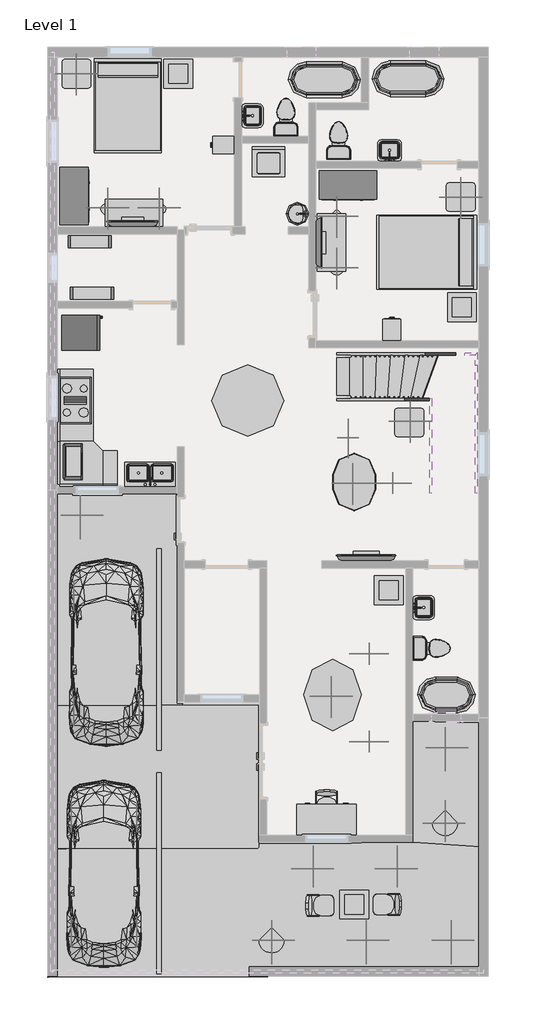
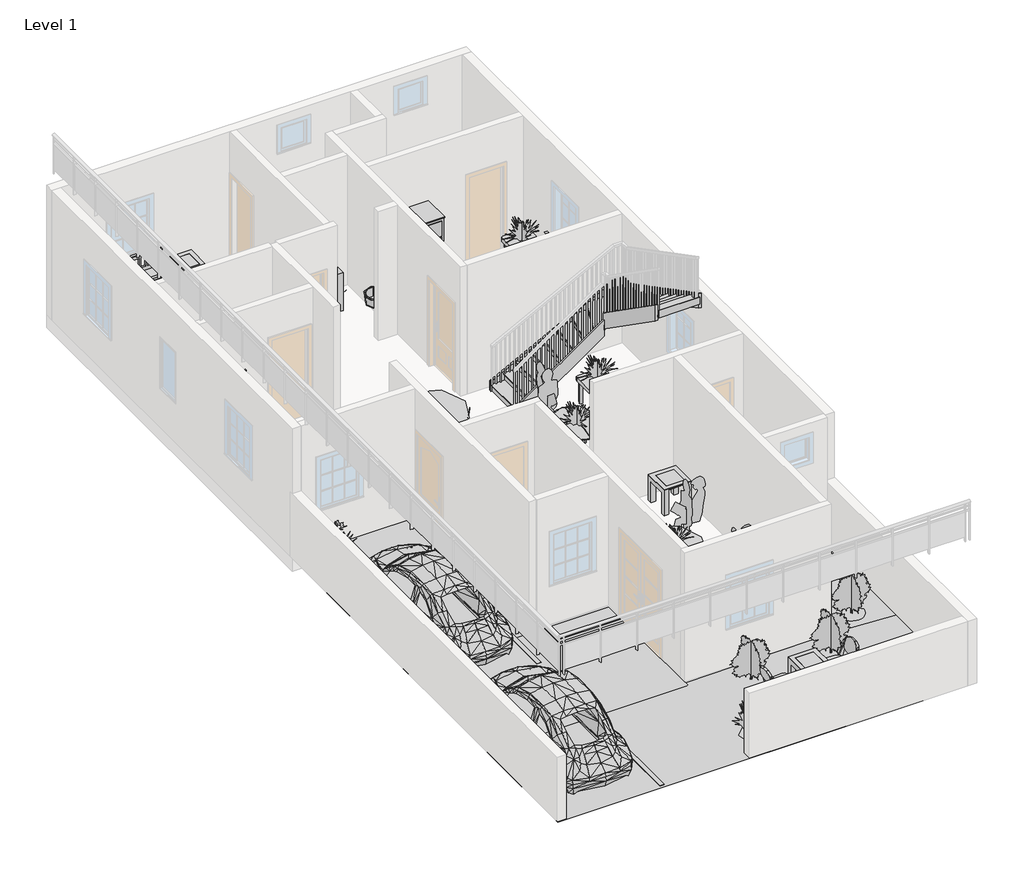
# One storey, part 4 of 4: 28 furniture elements, 17 geographic elements, 16 proxies, 15 flow terminals, 6 members, 1 stair flight.
"""IFC4 building model written with IfcOpenShell, lengths in millimetres."""

from ifc_helpers import new_model, si_unit, frame, origin, place, context, project, spatial, polyline, outline, extrude, triangles, transform, mapped, element, save
from components import proxy_bb1e6e30, proxy_8a8d5ab2, parking_space_9_x_18_90_deg_fdd9e8f5, rpc_beetle_rpc_beetle_3ce7ba48, rpc_female_69e001fa, proxy_a13a33b2, proxy_718fa39f, flow_terminal_accce45a, flow_terminal_a53be723, flow_terminal_d49f872f, flow_terminal_62a433f7, toilet_domestic_3d_toilet_domestic_3d_f7549cf7, toilet_domestic_3d_toilet_domestic_3d_183bbd19, flow_terminal_b374fae2, flow_terminal_04541809, furniture_096e7f55, furniture_35c09872, furniture_bb55ed6b, furniture_e086674a, furniture_9fa109b2, furniture_3d1d9cbc, furniture_417d203a, furniture_7a3aaa4f, furniture_fdf74506, furniture_b5c51a22, furniture_be1c6672, furniture_bbcc68ce, furniture_743965d2, furniture_31d08a24, furniture_9a1a9c00, furniture_823e54a9, rpc_plant_tropical_55f6ff97, rpc_plant_tropical_agave_1_5_93a2a214, rpc_plant_tropical_jungle_flame_3_9c4808c2, stair_flight_aca28aa2

model = new_model("IFC4")

# Units and contexts
model_context = context("Model", 3, world=origin())
ifc_project = project(units=[si_unit("LENGTHUNIT", "METRE", prefix="MILLI")], contexts=[model_context])

# Site, building, storey
site = spatial("IfcSite", under=ifc_project)
building = spatial("IfcBuilding", under=site)
storey = spatial("IfcBuildingStorey", under=building, Name="Level 1", Elevation=0.0)

# Proxies
placement = place(None, origin())
element("IfcBuildingElementProxy", 1, Name="Building Element Proxy", at=placement, inside=storey, context=model_context, shape_type="Tessellation", body=[
    triangles([(-11802.0982178, 4379.0271858, 0.0), (-9058.8976364, 4379.0271858, 0.0), (-9058.8976364, -27.872824, 0.0), (-11802.0982178, -114.4208502, 0.0), (-8906.4976364, -27.872824, 0.0), (-9058.2005859, -225.4422167, 0.0)], [[1, 4, 3], [3, 4, 6], [1, 3, 2], [3, 5, 2], [5, 3, 6]], closed=False),
])
element("IfcBuildingElementProxy", 2, Name="Building Element Proxy", at=placement, inside=storey, context=model_context, shape_type="Tessellation", body=[
    triangles([(-11802.0982178, -3160.0754265, 0.0), (-2454.8975395, -3120.3229111, 0.0), (-2454.8975395, -5857.1727173, 0.0), (-11802.0982178, -5882.5729111, 0.0), (-4069.6108978, -3091.2976479, 0.0), (-7295.5854996, -3097.5405807, 0.0), (-4055.0975395, -3012.3728142, 0.0), (-7312.4141235, -3043.6589859, 0.0)], [[1, 4, 6], [8, 6, 7], [6, 8, 1], [4, 3, 6], [3, 2, 5], [5, 7, 6], [7, 5, 2], [3, 5, 6]], closed=False),
])
element("IfcBuildingElementProxy", 3, Name="Building Element Proxy", at=placement, inside=storey, context=model_context, shape_type="Tessellation", body=[
    triangles([(-11598.8978302, -112.4571982, 0.0), (-11598.8978302, -3148.0770309, 0.0), (-7349.0310745, -187.3552247, 0.0), (-7347.7823135, -3140.2966919, 0.0), (-7321.6606522, -3122.5297531, 0.0), (-7318.9974426, -200.8658099, 0.0), (-7318.9974426, -97.6646782, 0.0)], [[2, 3, 1], [3, 2, 4], [1, 3, 7], [5, 6, 3], [7, 3, 6], [3, 4, 5]], closed=False),
])
element("IfcBuildingElementProxy", 4, Name="Building Element Proxy", at=placement, inside=storey, context=model_context, shape_type="Tessellation", body=[
    triangles([(-4055.0975395, -545.620911, 0.0), (-4051.521595, -3119.7002747, 0.0), (-2658.0976364, -3116.7074341, 0.0), (-2658.0976364, -530.6196465, 0.0), (-4055.0975395, -446.9728263, 0.0), (-2658.0976364, -481.4069527, 0.0)], [[6, 5, 1], [3, 1, 2], [4, 6, 1], [3, 4, 1]], closed=False),
])
proxy_shape = proxy_bb1e6e30(model_context)
element("IfcBuildingElementProxy", 5, Name="Cook Top-4 Unit : 36\" x 20\"", ObjectType="Cook Top-4 Unit : 36\" x 20\"", at=placement, inside=storey, context=model_context, shape_type="MappedRepresentation", body=[
    mapped(proxy_shape, transform((-11217.8976606, 6360.2271763, 0.0), x_axis=(0.0, 1.0, 0.0), y_axis=(-1.0, 0.0, 0.0), z_axis=(0.0, 0.0, 1.0))),
])
proxy_2_shape = proxy_8a8d5ab2(model_context)
element("IfcBuildingElementProxy", 6, Name="Microwave : 30\" x 16\" x 18\"", ObjectType="Microwave : 30\" x 16\" x 18\"", at=placement, inside=storey, context=model_context, shape_type="MappedRepresentation", body=[
    mapped(proxy_2_shape, transform((-11621.7781665, 4564.5342989, 0.0), x_axis=(0.0, 1.000000000000001, 0.0), y_axis=(-1.000000000000001, 0.0, 0.0), z_axis=(0.0, 0.0, 1.0))),
])
parking_space_9_x_18_90_deg_shape = parking_space_9_x_18_90_deg_fdd9e8f5(model_context)
element("IfcBuildingElementProxy", 7, Name="Parking Space : 9' x 18' - 90 deg", ObjectType="Parking Space : 9' x 18' - 90 deg", at=placement, inside=storey, context=model_context, shape_type="MappedRepresentation", body=[
    mapped(parking_space_9_x_18_90_deg_shape, transform((-9439.8976606, -1056.5728237, 0.0), x_axis=(-1.0000000000000004, 0.0, 0.0), y_axis=(0.0, -1.0000000000000004, 0.0), z_axis=(0.0, 0.0, 1.0))),
])
element("IfcBuildingElementProxy", 8, Name="Parking Space : 9' x 18' - 90 deg", ObjectType="Parking Space : 9' x 18' - 90 deg", at=placement, inside=storey, context=model_context, shape_type="MappedRepresentation", body=[
    mapped(parking_space_9_x_18_90_deg_shape, transform((-9439.8976606, -5806.3728237, 0.0), x_axis=(-1.0000000000000004, 0.0, 0.0), y_axis=(0.0, -1.0000000000000004, 0.0), z_axis=(0.0, 0.0, 1.0))),
])
rpc_beetle_rpc_beetle_shape = rpc_beetle_rpc_beetle_3ce7ba48(model_context)
element("IfcBuildingElementProxy", 9, Name="RPC Beetle : RPC Beetle", ObjectType="RPC Beetle : RPC Beetle", at=placement, inside=storey, context=model_context, shape_type="MappedRepresentation", body=[
    mapped(rpc_beetle_rpc_beetle_shape, transform((-10557.4976606, -218.3728237, 0.0), x_axis=(1.0, 0.0, 0.0), y_axis=(0.0, 1.0, 0.0), z_axis=(0.0, 0.0, 1.0))),
])
element("IfcBuildingElementProxy", 10, Name="RPC Beetle : RPC Beetle", ObjectType="RPC Beetle : RPC Beetle", at=placement, inside=storey, context=model_context, shape_type="MappedRepresentation", body=[
    mapped(rpc_beetle_rpc_beetle_shape, transform((-10608.2976606, -4917.3728237, 0.0), x_axis=(1.0, 0.0, 0.0), y_axis=(0.0, 1.0, 0.0), z_axis=(0.0, 0.0, 1.0))),
])
rpc_female_shape = rpc_female_69e001fa(model_context)
element("IfcBuildingElementProxy", 11, Name="RPC Female", ObjectType="RPC Female", at=placement, inside=storey, context=model_context, shape_type="MappedRepresentation", body=[
    mapped(rpc_female_shape, transform((-5134.5976606, 988.1271763, 0.0), x_axis=(0.0, -1.0000000000000007, 0.0), y_axis=(1.0000000000000007, 0.0, 0.0), z_axis=(0.0, 0.0, 1.0))),
])
element("IfcBuildingElementProxy", 12, Name="RPC Female", ObjectType="RPC Female", at=placement, inside=storey, context=model_context, shape_type="MappedRepresentation", body=[
    mapped(rpc_female_shape, transform((-5134.5976606, -878.7728237, 0.0), x_axis=(0.0, -1.0, 0.0), y_axis=(1.0, 0.0, 0.0), z_axis=(0.0, 0.0, 1.0))),
])
element("IfcBuildingElementProxy", 13, Name="RPC Female", ObjectType="RPC Female", at=placement, inside=storey, context=model_context, shape_type="MappedRepresentation", body=[
    mapped(rpc_female_shape, transform((-4645.6476606, 4607.6271763, 0.0), x_axis=(0.0, -1.0, 0.0), y_axis=(1.0, 0.0, 0.0), z_axis=(0.0, 0.0, 1.0))),
])
element("IfcBuildingElementProxy", 14, Name="RPC Female", ObjectType="RPC Female", at=placement, inside=storey, context=model_context, shape_type="MappedRepresentation", body=[
    mapped(rpc_female_shape, transform((-5426.6976606, 5407.7271763, 0.0), x_axis=(1.0, 0.0, 0.0), y_axis=(0.0, 1.0, 0.0), z_axis=(0.0, 0.0, 1.0))),
])
proxy_3_shape = proxy_a13a33b2(model_context)
element("IfcBuildingElementProxy", 15, Name="Refrigerator : 30\" x 32\" RH", ObjectType="Refrigerator : 30\" x 32\" RH", at=placement, inside=storey, context=model_context, shape_type="MappedRepresentation", body=[
    mapped(proxy_3_shape, transform((-11116.2976606, 7797.3032048, 0.0), x_axis=(0.0, 1.0000000000000002, 0.0), y_axis=(-1.0000000000000002, 0.0, 0.0), z_axis=(0.0, 0.0, 1.0))),
])
proxy_4_shape = proxy_718fa39f(model_context)
element("IfcBuildingElementProxy", 16, Name="Washer : 27\" x 25\" x 35\"", ObjectType="Washer : 27\" x 25\" x 35\"", at=placement, inside=storey, context=model_context, shape_type="MappedRepresentation", body=[
    mapped(proxy_4_shape, transform((-7536.2151291, 11148.3776115, 0.0), x_axis=(1.0, 0.0, 0.0), y_axis=(0.0, 1.0, 0.0), z_axis=(0.0, 0.0, 1.0))),
])

# Flow terminals
flow_terminal_shape = flow_terminal_accce45a(model_context)
element("IfcFlowTerminal", 17, ObjectType="Floor Drain - Round : 5\" Strainer - 2\" Drain", at=placement, inside=storey, context=model_context, shape_type="MappedRepresentation", body=[
    mapped(flow_terminal_shape, transform((-6798.2976606, 13523.0271763, 0.0), x_axis=(1.0, 0.0, 0.0), y_axis=(0.0, 1.0, 0.0), z_axis=(0.0, 0.0, 1.0))),
])
element("IfcFlowTerminal", 18, ObjectType="Floor Drain - Round : 5\" Strainer - 2\" Drain", at=placement, inside=storey, context=model_context, shape_type="MappedRepresentation", body=[
    mapped(flow_terminal_shape, transform((-4766.2976606, 12532.4271763, 0.0), x_axis=(1.0, 0.0, 0.0), y_axis=(0.0, 1.0, 0.0), z_axis=(0.0, 0.0, 1.0))),
])
element("IfcFlowTerminal", 19, ObjectType="Floor Drain - Round : 5\" Strainer - 2\" Drain", at=placement, inside=storey, context=model_context, shape_type="MappedRepresentation", body=[
    mapped(flow_terminal_shape, transform((-2785.0976606, 721.4271763, 0.0), x_axis=(1.0, 0.0, 0.0), y_axis=(0.0, 1.0, 0.0), z_axis=(0.0, 0.0, 1.0))),
])
element("IfcFlowTerminal", 20, ObjectType="Floor Drain - Round : 5\" Strainer - 2\" Drain", at=placement, inside=storey, context=model_context, shape_type="MappedRepresentation", body=[
    mapped(flow_terminal_shape, transform((-6434.6557206, 11712.7623112, 0.0), x_axis=(1.0, 0.0, 0.0), y_axis=(0.0, 1.0, 0.0), z_axis=(0.0, 0.0, 1.0))),
])
flow_terminal_2_shape = flow_terminal_a53be723(model_context)
element("IfcFlowTerminal", 21, ObjectType="Sink Kitchen-Double : 42\" x 21\"", at=placement, inside=storey, context=model_context, shape_type="MappedRepresentation", body=[
    mapped(flow_terminal_2_shape, transform((-9614.7084201, 4787.7725774, 0.0), x_axis=(-1.0000000000000004, 0.0, 0.0), y_axis=(0.0, -1.0000000000000004, 0.0), z_axis=(0.0, 0.0, 1.0))),
])
flow_terminal_3_shape = flow_terminal_d49f872f(model_context)
element("IfcFlowTerminal", 22, ObjectType="Sink Vanity-Round : 19\" x 19\"", at=placement, inside=storey, context=model_context, shape_type="MappedRepresentation", body=[
    mapped(flow_terminal_3_shape, transform((-6587.9921244, 10419.2789168, 0.0), x_axis=(0.0, -1.0, 0.0), y_axis=(1.0, 0.0, 0.0), z_axis=(0.0, 0.0, 1.0))),
])
flow_terminal_4_shape = flow_terminal_62a433f7(model_context)
element("IfcFlowTerminal", 23, ObjectType="Sink Vanity-Square : 20\" x 18\"", at=placement, inside=storey, context=model_context, shape_type="MappedRepresentation", body=[
    mapped(flow_terminal_4_shape, transform((-7507.1522595, 12389.7379357, 0.0), x_axis=(0.0, 1.0000000000000002, 0.0), y_axis=(-1.0000000000000002, 0.0, 0.0), z_axis=(0.0, 0.0, 1.0))),
])
element("IfcFlowTerminal", 24, ObjectType="Sink Vanity-Square : 20\" x 18\"", at=placement, inside=storey, context=model_context, shape_type="MappedRepresentation", body=[
    mapped(flow_terminal_4_shape, transform((-4534.2057813, 11620.3725774, 0.0), x_axis=(-1.0000000000000002, 0.0, 0.0), y_axis=(0.0, -1.0000000000000002, 0.0), z_axis=(0.0, 0.0, 1.0))),
])
element("IfcFlowTerminal", 25, ObjectType="Sink Vanity-Square : 20\" x 18\"", at=placement, inside=storey, context=model_context, shape_type="MappedRepresentation", body=[
    mapped(flow_terminal_4_shape, transform((-3874.9522595, 1950.3379357, 0.0), x_axis=(0.0, 1.0000000000000002, 0.0), y_axis=(-1.0000000000000002, 0.0, 0.0), z_axis=(0.0, 0.0, 1.0))),
])
toilet_domestic_3d_toilet_domestic_3d_shape = toilet_domestic_3d_toilet_domestic_3d_f7549cf7(model_context)
toilet_domestic_3d_toilet_domestic_3d_2_shape = toilet_domestic_3d_toilet_domestic_3d_183bbd19(model_context)
element("IfcFlowTerminal", 26, ObjectType="Toilet-Domestic-3D : Toilet-Domestic-3D", at=placement, inside=storey, context=model_context, shape_type="MappedRepresentation", body=[
    mapped(toilet_domestic_3d_toilet_domestic_3d_shape, transform((-6747.4976606, 12468.3232036, 0.0), x_axis=(-1.0000000000000002, 0.0, 0.0), y_axis=(0.0, -1.0000000000000002, 0.0), z_axis=(0.0, 0.0, 1.0))),
    mapped(toilet_domestic_3d_toilet_domestic_3d_2_shape, transform((-6747.4976606, 12468.3232036, 0.0), x_axis=(-1.0000000000000002, 0.0, 0.0), y_axis=(0.0, -1.0000000000000002, 0.0), z_axis=(0.0, 0.0, 1.0))),
])
element("IfcFlowTerminal", 27, ObjectType="Toilet-Domestic-3D : Toilet-Domestic-3D", at=placement, inside=storey, context=model_context, shape_type="MappedRepresentation", body=[
    mapped(toilet_domestic_3d_toilet_domestic_3d_shape, transform((-5629.8976606, 11973.6271763, 0.0), x_axis=(-1.0, 0.0, 0.0), y_axis=(0.0, -1.0, 0.0), z_axis=(0.0, 0.0, 1.0))),
    mapped(toilet_domestic_3d_toilet_domestic_3d_2_shape, transform((-5629.8976606, 11973.6271763, 0.0), x_axis=(-1.0, 0.0, 0.0), y_axis=(0.0, -1.0, 0.0), z_axis=(0.0, 0.0, 1.0))),
])
element("IfcFlowTerminal", 28, ObjectType="Toilet-Domestic-3D : Toilet-Domestic-3D", at=placement, inside=storey, context=model_context, shape_type="MappedRepresentation", body=[
    mapped(toilet_domestic_3d_toilet_domestic_3d_shape, transform((-3560.4016333, 1102.4271763, 0.0), x_axis=(0.0, 1.0000000000000002, 0.0), y_axis=(-1.0000000000000002, 0.0, 0.0), z_axis=(0.0, 0.0, 1.0))),
    mapped(toilet_domestic_3d_toilet_domestic_3d_2_shape, transform((-3560.4016333, 1102.4271763, 0.0), x_axis=(0.0, 1.0000000000000002, 0.0), y_axis=(-1.0000000000000002, 0.0, 0.0), z_axis=(0.0, 0.0, 1.0))),
])
flow_terminal_5_shape = flow_terminal_b374fae2(model_context)
element("IfcFlowTerminal", 29, ObjectType="Tub-Free Standing-3D : 30\" x 60\"", at=placement, inside=storey, context=model_context, shape_type="MappedRepresentation", body=[
    mapped(flow_terminal_5_shape, transform((-5934.6976606, 13167.4271763, 0.0), x_axis=(0.0, -1.0000000000000002, 0.0), y_axis=(1.0000000000000002, 0.0, 0.0), z_axis=(0.0, 0.0, 1.0))),
])
element("IfcFlowTerminal", 30, ObjectType="Tub-Free Standing-3D : 30\" x 60\"", at=placement, inside=storey, context=model_context, shape_type="MappedRepresentation", body=[
    mapped(flow_terminal_5_shape, transform((-4156.6976606, 13192.8271763, 0.0), x_axis=(0.0, 1.0, 0.0), y_axis=(-1.0, 0.0, 0.0), z_axis=(0.0, 0.0, 1.0))),
])
flow_terminal_6_shape = flow_terminal_04541809(model_context)
element("IfcFlowTerminal", 31, ObjectType="Tub-Free Standing-3D : 30\" x 60\" 2", at=placement, inside=storey, context=model_context, shape_type="MappedRepresentation", body=[
    mapped(flow_terminal_6_shape, transform((-3343.8976606, 111.8271763, 0.0), x_axis=(0.0, 1.0, 0.0), y_axis=(-1.0, 0.0, 0.0), z_axis=(0.0, 0.0, 1.0))),
])

# Furniture
furniture_shape = furniture_096e7f55(model_context)
element("IfcFurniture", 32, ObjectType="Bed-Shaker : Double 56\" x 78\"", at=placement, inside=storey, context=model_context, shape_type="MappedRepresentation", body=[
    mapped(furniture_shape, transform((-10081.2476606, 13599.2271763, 0.0), x_axis=(1.0, 0.0, 0.0), y_axis=(0.0, 1.0, 0.0), z_axis=(0.0, 0.0, 1.0))),
])
furniture_2_shape = furniture_35c09872(model_context)
element("IfcFurniture", 33, ObjectType="Bed-Shaker : Queen 62\" x 83\"", at=placement, inside=storey, context=model_context, shape_type="MappedRepresentation", body=[
    mapped(furniture_2_shape, transform((-2708.8976606, 9490.7771763, 0.0), x_axis=(0.0, -0.9999999999999998, 0.0), y_axis=(0.9999999999999998, 0.0, 0.0), z_axis=(0.0, 0.0, 1.0))),
])
furniture_3_shape = furniture_bb55ed6b(model_context)
element("IfcFurniture", 34, ObjectType="Cabinet-File 2 Drawer : 15\" x 18\"", at=placement, inside=storey, context=model_context, shape_type="MappedRepresentation", body=[
    mapped(furniture_3_shape, transform((-7926.1633605, 11655.2307292, 0.0), x_axis=(0.0, -0.9999999999999998, 0.0), y_axis=(0.9999999999999998, 0.0, 0.0), z_axis=(0.0, 0.0, 1.0))),
])
element("IfcFurniture", 35, ObjectType="Cabinet-File 2 Drawer : 15\" x 18\"", at=placement, inside=storey, context=model_context, shape_type="MappedRepresentation", body=[
    mapped(furniture_3_shape, transform((-4627.4941077, 7716.6928761, 0.0), x_axis=(-0.9999999999999998, 0.0, 0.0), y_axis=(0.0, -0.9999999999999998, 0.0), z_axis=(0.0, 0.0, 1.0))),
])
furniture_4_shape = furniture_e086674a(model_context)
element("IfcFurniture", 36, ObjectType="Desk : 60\" x 30\" Student", at=placement, inside=storey, context=model_context, shape_type="MappedRepresentation", body=[
    mapped(furniture_4_shape, transform((-5121.8976606, -2148.7728237, 0.0), x_axis=(-1.0000000000000004, 0.0, 0.0), y_axis=(0.0, -1.0000000000000004, 0.0), z_axis=(0.0, 0.0, 1.0))),
])
furniture_5_shape = furniture_9fa109b2(model_context)
element("IfcFurniture", 37, ObjectType="Dresser : 48\" x 72\" x 24\"", at=placement, inside=storey, context=model_context, shape_type="MappedRepresentation", body=[
    mapped(furniture_5_shape, transform((-11606.4606147, 10972.8204361, 0.0), x_axis=(0.0, 1.0000000000000002, 0.0), y_axis=(-1.0000000000000002, 0.0, 0.0), z_axis=(0.0, 0.0, 1.0))),
])
element("IfcFurniture", 38, ObjectType="Dresser : 48\" x 72\" x 24\"", at=placement, inside=storey, context=model_context, shape_type="MappedRepresentation", body=[
    mapped(furniture_5_shape, transform((-5157.5044008, 11295.3901304, 0.0), x_axis=(1.0, 0.0, 0.0), y_axis=(0.0, 1.0, 0.0), z_axis=(0.0, 0.0, 1.0))),
])
furniture_6_shape = furniture_3d1d9cbc(model_context)
element("IfcFurniture", 39, ObjectType="Seating-Auditorium : 18\" x 24\" x 30\"", at=placement, inside=storey, context=model_context, shape_type="MappedRepresentation", body=[
    mapped(furniture_6_shape, transform((-5723.1697918, -1996.9974139, 0.0), x_axis=(-1.0000000000000004, 0.0, 0.0), y_axis=(0.0, -1.0000000000000004, 0.0), z_axis=(0.0, 0.0, 1.0))),
])
element("IfcFurniture", 40, ObjectType="Seating-Auditorium : 18\" x 24\" x 30\"", at=placement, inside=storey, context=model_context, shape_type="MappedRepresentation", body=[
    mapped(furniture_6_shape, transform((-6226.1730705, -4197.8449549, 0.0), x_axis=(0.0, -1.0000000000000007, 0.0), y_axis=(1.0000000000000007, 0.0, 0.0), z_axis=(0.0, 0.0, 1.0))),
])
element("IfcFurniture", 41, ObjectType="Seating-Auditorium : 18\" x 24\" x 30\"", at=placement, inside=storey, context=model_context, shape_type="MappedRepresentation", body=[
    mapped(furniture_6_shape, transform((-4398.6222508, -4493.9006926, 0.0), x_axis=(0.0, 1.000000000000001, 0.0), y_axis=(-1.000000000000001, 0.0, 0.0), z_axis=(0.0, 0.0, 1.0))),
])
furniture_7_shape = furniture_417d203a(model_context)
element("IfcFurniture", 42, ObjectType="Shelving : 36\" x 10\" x 72\"", at=placement, inside=storey, context=model_context, shape_type="MappedRepresentation", body=[
    mapped(furniture_7_shape, transform((-10913.0976606, 9420.9271763, 0.0), x_axis=(-1.0, 0.0, 0.0), y_axis=(0.0, -1.0, 0.0), z_axis=(0.0, 0.0, 1.0))),
])
element("IfcFurniture", 43, ObjectType="Shelving : 36\" x 10\" x 72\"", at=placement, inside=storey, context=model_context, shape_type="MappedRepresentation", body=[
    mapped(furniture_7_shape, transform((-10862.2976606, 8335.0771763, 0.0), x_axis=(-1.0000000000000004, 0.0, 0.0), y_axis=(0.0, -1.0000000000000004, 0.0), z_axis=(0.0, 0.0, 1.0))),
])
furniture_8_shape = furniture_7a3aaa4f(model_context)
element("IfcFurniture", 44, ObjectType="TV - Flat Screen : 42\"", at=placement, inside=storey, context=model_context, shape_type="MappedRepresentation", body=[
    mapped(furniture_8_shape, transform((-10002.6421748, 10101.7657999, 1041.4), x_axis=(-0.9999999999999998, 0.0, 0.0), y_axis=(0.0, -0.9999999999999998, 0.0), z_axis=(0.0, 0.0, 1.0))),
])
element("IfcFurniture", 45, ObjectType="TV - Flat Screen : 42\"", at=placement, inside=storey, context=model_context, shape_type="MappedRepresentation", body=[
    mapped(furniture_8_shape, transform((-6053.959037, 9716.9716904, 1041.4), x_axis=(0.0, 1.0000000000000002, 0.0), y_axis=(-1.0000000000000002, 0.0, 0.0), z_axis=(0.0, 0.0, 1.0))),
])
furniture_9_shape = furniture_fdf74506(model_context)
element("IfcFurniture", 46, ObjectType="TV - Flat Screen : 50\"", at=placement, inside=storey, context=model_context, shape_type="MappedRepresentation", body=[
    mapped(furniture_9_shape, transform((-5049.6421748, 3015.1657999, 1041.4), x_axis=(-1.0000000000000002, 0.0, 0.0), y_axis=(0.0, -1.0000000000000002, 0.0), z_axis=(0.0, 0.0, 1.0))),
])
furniture_10_shape = furniture_b5c51a22(model_context)
element("IfcFurniture", 47, ObjectType="Table-Coffee : 24\" x 24\" x 24\"", at=placement, inside=storey, context=model_context, shape_type="MappedRepresentation", body=[
    mapped(furniture_10_shape, transform((-9051.7634273, 13199.2160985, 0.0), x_axis=(1.0, 0.0, 0.0), y_axis=(0.0, 1.0, 0.0), z_axis=(0.0, 0.0, 1.0))),
])
element("IfcFurniture", 48, ObjectType="Table-Coffee : 24\" x 24\" x 24\"", at=placement, inside=storey, context=model_context, shape_type="MappedRepresentation", body=[
    mapped(furniture_10_shape, transform((-3031.9634273, 8246.2160985, 0.0), x_axis=(1.0, 0.0, 0.0), y_axis=(0.0, 1.0, 0.0), z_axis=(0.0, 0.0, 1.0))),
])
element("IfcFurniture", 49, ObjectType="Table-Coffee : 24\" x 24\" x 24\"", at=placement, inside=storey, context=model_context, shape_type="MappedRepresentation", body=[
    mapped(furniture_10_shape, transform((-4581.3634273, 2239.1160985, 0.0), x_axis=(1.0, 0.0, 0.0), y_axis=(0.0, 1.0, 0.0), z_axis=(0.0, 0.0, 1.0))),
])
element("IfcFurniture", 50, ObjectType="Table-Coffee : 24\" x 24\" x 24\"", at=placement, inside=storey, context=model_context, shape_type="MappedRepresentation", body=[
    mapped(furniture_10_shape, transform((-5317.9634273, -4428.3839015, 0.0), x_axis=(1.0, 0.0, 0.0), y_axis=(0.0, 1.0, 0.0), z_axis=(0.0, 0.0, 1.0))),
])
furniture_11_shape = furniture_be1c6672(model_context)
element("IfcFurniture", 51, ObjectType="Table-Dining Oval : 36\" x 48\"", at=placement, inside=storey, context=model_context, shape_type="MappedRepresentation", body=[
    mapped(furniture_11_shape, transform((-5657.7960213, 5034.8468484, 0.0), x_axis=(0.0, 1.0000000000000002, 0.0), y_axis=(-1.0000000000000002, 0.0, 0.0), z_axis=(0.0, 0.0, 1.0))),
])
furniture_12_shape = furniture_bbcc68ce(model_context)
element("IfcFurniture", 52, ObjectType="Table-Dining Round w Chairs : 60\" Diameter", at=placement, inside=storey, context=model_context, shape_type="MappedRepresentation", body=[
    mapped(furniture_12_shape, transform((-7663.9796279, 6545.1058648, 0.0), x_axis=(1.0, 0.0, 0.0), y_axis=(0.0, 1.0, 0.0), z_axis=(0.0, 0.0, 1.0))),
])
furniture_13_shape = furniture_743965d2(model_context)
element("IfcFurniture", 53, ObjectType="Table-Ellipse : 60\" x 48\"", at=placement, inside=storey, context=model_context, shape_type="MappedRepresentation", body=[
    mapped(furniture_13_shape, transform((-5756.8976606, 111.8271763, 0.0), x_axis=(0.0, 1.0, 0.0), y_axis=(-1.0, 0.0, 0.0), z_axis=(0.0, 0.0, 1.0))),
])
furniture_14_shape = furniture_31d08a24(model_context)
element("IfcFurniture", 54, ObjectType="Table-End : 24\" x 24\"", at=placement, inside=storey, context=model_context, shape_type="MappedRepresentation", body=[
    mapped(furniture_14_shape, transform((-11501.0312909, 13142.0271763, 0.0), x_axis=(1.0, 0.0, 0.0), y_axis=(0.0, 1.0, 0.0), z_axis=(0.0, 0.0, 1.0))),
])
element("IfcFurniture", 55, ObjectType="Table-End : 24\" x 24\"", at=placement, inside=storey, context=model_context, shape_type="MappedRepresentation", body=[
    mapped(furniture_14_shape, transform((-3347.6312909, 10525.8271763, 0.0), x_axis=(1.0, 0.0, 0.0), y_axis=(0.0, 1.0, 0.0), z_axis=(0.0, 0.0, 1.0))),
])
element("IfcFurniture", 56, ObjectType="Table-End : 24\" x 24\"", at=placement, inside=storey, context=model_context, shape_type="MappedRepresentation", body=[
    mapped(furniture_14_shape, transform((-4439.8312909, 5744.2771763, 0.0), x_axis=(1.0, 0.0, 0.0), y_axis=(0.0, 1.0, 0.0), z_axis=(0.0, 0.0, 1.0))),
])
furniture_15_shape = furniture_9a1a9c00(model_context)
element("IfcFurniture", 57, ObjectType="Table-Rectangular : 72\" x 30\"", at=placement, inside=storey, context=model_context, shape_type="MappedRepresentation", body=[
    mapped(furniture_15_shape, transform((-9973.2976606, 10322.6271763, 0.0), x_axis=(1.0, 0.0, 0.0), y_axis=(0.0, 1.0, 0.0), z_axis=(0.0, 0.0, 1.0))),
])
element("IfcFurniture", 58, ObjectType="Table-Rectangular : 72\" x 30\"", at=placement, inside=storey, context=model_context, shape_type="MappedRepresentation", body=[
    mapped(furniture_15_shape, transform((-5782.2976606, 9713.0271763, 0.0), x_axis=(0.0, 1.0, 0.0), y_axis=(-1.0, 0.0, 0.0), z_axis=(0.0, 0.0, 1.0))),
])
furniture_16_shape = furniture_823e54a9(model_context)
element("IfcFurniture", 59, ObjectType="Work Station Cubicle : 96\" x 96\"", at=placement, inside=storey, context=model_context, shape_type="MappedRepresentation", body=[
    mapped(furniture_16_shape, transform((-12093.9206683, 4663.1589285, 0.0), x_axis=(0.0, 0.9999999999999999, 0.0), y_axis=(-0.9999999999999999, 0.0, 0.0), z_axis=(0.0, 0.0, 1.0))),
])

# Geographic elements
rpc_plant_tropical_shape = rpc_plant_tropical_55f6ff97(model_context)
element("IfcGeographicElement", 60, ObjectType="RPC Plant - Tropical", at=placement, inside=storey, context=model_context, shape_type="MappedRepresentation", body=[
    mapped(rpc_plant_tropical_shape, transform((-11116.2976606, 3921.8271763, 0.0), x_axis=(1.0, 0.0, 0.0), y_axis=(0.0, 1.0, 0.0), z_axis=(0.0, 0.0, 1.0))),
])
element("IfcGeographicElement", 61, ObjectType="RPC Plant - Tropical", at=placement, inside=storey, context=model_context, shape_type="MappedRepresentation", body=[
    mapped(rpc_plant_tropical_shape, transform((-3242.2976606, -5095.1728237, 0.0), x_axis=(1.0, 0.0, 0.0), y_axis=(0.0, 1.0, 0.0), z_axis=(0.0, 0.0, 1.0))),
])
element("IfcGeographicElement", 62, ObjectType="RPC Plant - Tropical", at=placement, inside=storey, context=model_context, shape_type="MappedRepresentation", body=[
    mapped(rpc_plant_tropical_shape, transform((-5045.6976606, -5095.1728237, 0.0), x_axis=(1.0, 0.0, 0.0), y_axis=(0.0, 1.0, 0.0), z_axis=(0.0, 0.0, 1.0))),
])
element("IfcGeographicElement", 63, ObjectType="RPC Plant - Tropical", at=placement, inside=storey, context=model_context, shape_type="MappedRepresentation", body=[
    mapped(rpc_plant_tropical_shape, transform((-7052.2976606, -5095.1728237, 0.0), x_axis=(1.0, 0.0, 0.0), y_axis=(0.0, 1.0, 0.0), z_axis=(0.0, 0.0, 1.0))),
])
element("IfcGeographicElement", 64, ObjectType="RPC Plant - Tropical", at=placement, inside=storey, context=model_context, shape_type="MappedRepresentation", body=[
    mapped(rpc_plant_tropical_shape, transform((-3369.2976606, -1005.7728237, 0.0), x_axis=(1.0, 0.0, 0.0), y_axis=(0.0, 1.0, 0.0), z_axis=(0.0, 0.0, 1.0))),
])
rpc_plant_tropical_agave_1_5_shape = rpc_plant_tropical_agave_1_5_93a2a214(model_context)
element("IfcGeographicElement", 65, ObjectType="RPC Plant - Tropical : Agave - 1.5'", at=placement, inside=storey, context=model_context, shape_type="MappedRepresentation", body=[
    mapped(rpc_plant_tropical_agave_1_5_shape, transform((-11192.4976606, 13294.4271763, 609.6), x_axis=(1.0, 0.0, 0.0), y_axis=(0.0, 1.0, 0.0), z_axis=(0.0, 0.0, 1.0))),
])
element("IfcGeographicElement", 66, ObjectType="RPC Plant - Tropical : Agave - 1.5'", at=placement, inside=storey, context=model_context, shape_type="MappedRepresentation", body=[
    mapped(rpc_plant_tropical_agave_1_5_shape, transform((-3039.0976606, 10678.2271763, 609.6), x_axis=(1.0, 0.0, 0.0), y_axis=(0.0, 1.0, 0.0), z_axis=(0.0, 0.0, 1.0))),
])
element("IfcGeographicElement", 67, ObjectType="RPC Plant - Tropical : Agave - 1.5'", at=placement, inside=storey, context=model_context, shape_type="MappedRepresentation", body=[
    mapped(rpc_plant_tropical_agave_1_5_shape, transform((-5325.0976606, 4607.6271763, 736.6), x_axis=(1.0, 0.0, 0.0), y_axis=(0.0, 1.0, 0.0), z_axis=(0.0, 0.0, 1.0))),
])
element("IfcGeographicElement", 68, ObjectType="RPC Plant - Tropical : Agave - 1.5'", at=placement, inside=storey, context=model_context, shape_type="MappedRepresentation", body=[
    mapped(rpc_plant_tropical_agave_1_5_shape, transform((-4105.8976606, 5922.0771763, 609.6), x_axis=(1.0, 0.0, 0.0), y_axis=(0.0, 1.0, 0.0), z_axis=(0.0, 0.0, 1.0))),
])
element("IfcGeographicElement", 69, ObjectType="RPC Plant - Tropical : Agave - 1.5'", at=placement, inside=storey, context=model_context, shape_type="MappedRepresentation", body=[
    mapped(rpc_plant_tropical_agave_1_5_shape, transform((-5782.2976606, 86.4271763, 762.0), x_axis=(1.0, 0.0, 0.0), y_axis=(0.0, 1.0, 0.0), z_axis=(0.0, 0.0, 1.0))),
])
element("IfcGeographicElement", 70, ObjectType="RPC Plant - Tropical : Agave - 1.5'", at=placement, inside=storey, context=model_context, shape_type="MappedRepresentation", body=[
    mapped(rpc_plant_tropical_agave_1_5_shape, transform((-9439.8976606, 10449.6271763, 609.6), x_axis=(1.0, 0.0, 0.0), y_axis=(0.0, 1.0, 0.0), z_axis=(0.0, 0.0, 1.0))),
])
element("IfcGeographicElement", 71, ObjectType="RPC Plant - Tropical : Agave - 1.5'", at=placement, inside=storey, context=model_context, shape_type="MappedRepresentation", body=[
    mapped(rpc_plant_tropical_agave_1_5_shape, transform((-10532.0976606, 10449.6271763, 609.6), x_axis=(1.0, 0.0, 0.0), y_axis=(0.0, 1.0, 0.0), z_axis=(0.0, 0.0, 1.0))),
])
element("IfcGeographicElement", 72, ObjectType="RPC Plant - Tropical : Agave - 1.5'", at=placement, inside=storey, context=model_context, shape_type="MappedRepresentation", body=[
    mapped(rpc_plant_tropical_agave_1_5_shape, transform((-5667.9976606, 10271.8271763, 609.6), x_axis=(1.0, 0.0, 0.0), y_axis=(0.0, 1.0, 0.0), z_axis=(0.0, 0.0, 1.0))),
])
element("IfcGeographicElement", 73, ObjectType="RPC Plant - Tropical : Agave - 1.5'", at=placement, inside=storey, context=model_context, shape_type="MappedRepresentation", body=[
    mapped(rpc_plant_tropical_agave_1_5_shape, transform((-5667.9976606, 9179.6271763, 609.6), x_axis=(1.0, 0.0, 0.0), y_axis=(0.0, 1.0, 0.0), z_axis=(0.0, 0.0, 1.0))),
])
rpc_plant_tropical_jungle_flame_3_shape = rpc_plant_tropical_jungle_flame_3_9c4808c2(model_context)
element("IfcGeographicElement", 74, ObjectType="RPC Plant - Tropical : Jungle Flame - 3'", at=placement, inside=storey, context=model_context, shape_type="MappedRepresentation", body=[
    mapped(rpc_plant_tropical_jungle_flame_3_shape, transform((-6163.2976606, -3571.1728237, 0.0), x_axis=(1.0, 0.0, 0.0), y_axis=(0.0, 1.0, 0.0), z_axis=(0.0, 0.0, 1.0))),
])
element("IfcGeographicElement", 75, ObjectType="RPC Plant - Tropical : Jungle Flame - 3'", at=placement, inside=storey, context=model_context, shape_type="MappedRepresentation", body=[
    mapped(rpc_plant_tropical_jungle_flame_3_shape, transform((-4385.2976606, -3571.1728237, 0.0), x_axis=(1.0, 0.0, 0.0), y_axis=(0.0, 1.0, 0.0), z_axis=(0.0, 0.0, 1.0))),
])
element("IfcGeographicElement", 76, ObjectType="RPC Plant - Tropical : Jungle Flame - 3'", at=placement, inside=storey, context=model_context, shape_type="MappedRepresentation", body=[
    mapped(rpc_plant_tropical_jungle_flame_3_shape, transform((-3369.2976606, -2605.9728237, 0.0), x_axis=(1.0, 0.0, 0.0), y_axis=(0.0, 1.0, 0.0), z_axis=(0.0, 0.0, 1.0))),
])

# Members
element("IfcMember", 77, ObjectType="Stringer - 2\" Width", at=placement, inside=storey, context=model_context, shape_type="SweptSolid", body=[
    extrude(outline(polyline([(228.5422831, -5670.2346501), (0.0, -5670.2346501), (0.0, -5449.2024483), (1300.4000987, -2952.4510037), (1644.0640924, -2952.4510037), (228.5422831, -5670.2346501)])), frame((0.0, 7325.4271763, 0.0), z_axis=(0.0, 1.0, 0.0), x_axis=(0.0, 0.0, 1.0)), (0.0, 0.0, 1.0), 50.8),
])
element("IfcMember", 78, ObjectType="Stringer - 2\" Width", at=placement, inside=storey, context=model_context, shape_type="SweptSolid", body=[
    extrude(outline(polyline([(-2952.4510037, 7325.4271763), (-2952.4510037, 7376.2271763), (-2683.4976606, 7376.2271763), (-2734.2976606, 7325.4271763), (-2952.4510037, 7325.4271763)])), frame((0.0, 0.0, 1300.4000987), z_axis=(0.0, 0.0, 1.0), x_axis=(1.0, 0.0, 0.0)), (0.0, 0.0, 1.0), 343.6639937),
])
element("IfcMember", 79, ObjectType="Stringer - 2\" Width", at=placement, inside=storey, context=model_context, shape_type="SweptSolid", body=[
    extrude(outline(polyline([(-2734.2976606, 7325.4271763), (-2683.4976606, 7376.2271763), (-2683.4976606, 7107.2738332), (-2734.2976606, 7107.2738332), (-2734.2976606, 7325.4271763)])), frame((0.0, 0.0, 1300.4000987), z_axis=(0.0, 0.0, 1.0), x_axis=(1.0, 0.0, 0.0)), (0.0, 0.0, 1.0), 343.6639937),
])
element("IfcMember", 80, ObjectType="Stringer - 2\" Width", at=placement, inside=storey, context=model_context, shape_type="SweptSolid", body=[
    extrude(outline(polyline([(7107.2738332, 1644.0640924), (7107.2738332, 1300.4000987), (4389.4901868, 2715.921908), (4389.4901868, 3059.5859017), (7107.2738332, 1644.0640924)])), frame((-2734.2976606, 0.0, 0.0), z_axis=(1.0, 0.0, 0.0), x_axis=(0.0, 1.0, 0.0)), (0.0, 0.0, 1.0), 50.8),
])
element("IfcMember", 81, ObjectType="Stringer - 2\" Width", at=placement, inside=storey, context=model_context, shape_type="SweptSolid", body=[
    extrude(outline(polyline([(195.121823, -5670.2346501), (0.0, -5670.2346501), (0.0, -5417.56878), (1204.1488295, -3699.4976606), (1576.3572168, -3699.4976606), (195.121823, -5670.2346501)])), frame((0.0, 6360.2271763, 0.0), z_axis=(0.0, 1.0, 0.0), x_axis=(0.0, 0.0, 1.0)), (0.0, 0.0, 1.0), 50.8),
])
element("IfcMember", 82, ObjectType="Stringer - 2\" Width", at=placement, inside=storey, context=model_context, shape_type="SweptSolid", body=[
    extrude(outline(polyline([(6411.0271763, 1709.9296678), (6411.0271763, 1337.7212805), (4389.4901868, 2754.5609981), (4389.4901868, 3126.7693854), (6411.0271763, 1709.9296678)])), frame((-3699.4976606, 0.0, 0.0), z_axis=(1.0, 0.0, 0.0), x_axis=(0.0, 1.0, 0.0)), (0.0, 0.0, 1.0), 50.8),
])

# Stair flight
stair_flight_shape = stair_flight_aca28aa2(model_context)
element("IfcStairFlight", 83, ObjectType="2\" Tread 1\" Nosing 1/4\" Riser", at=placement, inside=storey, context=model_context, shape_type="MappedRepresentation", body=[
    mapped(stair_flight_shape, transform((0.0, 0.0, 0.0), x_axis=(1.0, 0.0, 0.0), y_axis=(0.0, 1.0, 0.0), z_axis=(0.0, 0.0, 1.0))),
])

save(model, "model.ifc")

# Revit data of these elements
# Type "Cook Top-4 Unit : 36\" x 20\""
#   Assembly Code = "E1090400"
#   Depth = 2' - 0"
#   Width = 3' - 0"
#   Burner Material = Steel, Chrome Plated
#   Cooktop Material = Steel, Polished
#   Default Elevation = 0
# Type "Microwave : 30\" x 16\" x 18\""
#   Assembly Code = "E1090400"
#   Depth = 1' - 4"
#   Height = 1' - 6"
#   Width = 2' - 6"
#   Microwave Material = Laminate, Linen, Matte
#   Default Elevation = 0
# Type "Parking Space : 9' x 18' - 90 deg"
#   Angle = 90.00°
#   Parking Length = 18' - 0"
#   Parking Width = 9' - 0"
#   pl = 14' - 0"
#   pw = 7' - 0"
# Type "RPC Beetle : RPC Beetle"
#   built-in parameter 1005195 = "RPC-16-0U6E-L4EG-ENH1-J3KF-SVEL-0TX4-C0"
#   Height = 0
# Type "RPC Female"
#   built-in parameter 1005195 = "RPC-8-FXA2-QQQ0-UGV2-6"
#   Height = 0
# Type "Refrigerator : 30\" x 32\" RH"
#   Label = "REF."
#   Assembly Code = "E1090400"
#   Depth = 2' - 7 3/4"
#   Handle = 2' - 3"
#   Height = 5' - 10"
#   Rear Clearance = 0' - 2"
#   Top Door Height = 1' - 8"
#   Width = 2' - 5 3/8"
#   Material = Carpet (1)
#   Default Elevation = 0
# Type "Washer : 27\" x 25\" x 35\""
#   Label = "W"
#   Assembly Code = "E1090400"
#   Depth = 2' - 1"
#   Height = 2' - 11"
#   Width = 2' - 3"
#   Washer Material = Steel, Paint Finish, Ivory, Matte
#   Default Elevation = 0
# Type "Floor Drain - Round : 5\" Strainer - 2\" Drain"
#   WFU = 2
#   Strainer Height = 0' - 3 1/4"
#   Strainer Radius = 0' - 2 1/2"
#   Strainer Diameter = 0' - 5"
#   Radius 6 = 0' - 0 5/8"
#   Radius 5 = 0' - 1 1/4"
#   Radius 4 = 0' - 1 7/8"
#   Radius 2 = 0' - 3.04167"
#   Radius 1 = 0' - 2.02083"
#   Radius 3 = 0' - 2 1/32"
#   Pipe Radius = 1"
#   Pipe Diameter = 2"
#   Height 2 = 0' - 0.725"
#   Height 1 = 0' - 1 13/16"
#   Body Radius = 0' - 4 1/16"
#   Body Height = 0' - 3 5/8"
#   Body Diameter = 0' - 8 1/8"
#   Drain Material = none
#   HWFU = 0
#   Default Elevation = 0
#   CWFU = 0
# Type "Sink Kitchen-Double : 42\" x 21\""
#   Assembly Code = "D2010410"
#   Counter Height = 3' - 0"
#   Depth = 1' - 9"
#   Width = 3' - 6"
#   Faucet Material = Steel, Polished
#   Sink Material = Steel, Polished
#   Default Elevation = 0
# Type "Sink Vanity-Round : 19\" x 19\""
#   Assembly Code = "D2010400"
#   Top Of Counter = 2' - 7"
#   Basin Material = Porcelain, Linen
#   Faucet Material = Steel, Polished
#   Default Elevation = 0
# Type "Sink Vanity-Square : 20\" x 18\""
#   Assembly Code = "D2010400"
#   Counter Height = 2' - 7"
#   Depth = 1' - 6"
#   Width = 1' - 8"
#   Basin Material = Porcelain, Linen
#   Faucet Material = Steel, Polished
#   Default Elevation = 0
# Type "Toilet-Domestic-3D : Toilet-Domestic-3D"
#   Assembly Code = "D2010110"
#   Toilet - Bowl/Basin Material = Porcelain, Linen
#   Toilet - Seat Material = Laminate, Linen, Matte
#   Default Elevation = 0
# Type "Tub-Free Standing-3D : 30\" x 60\""
#   Assembly Code = "D2010110"
#   Height = 1' - 6"
#   Length = 5' - 0"
#   Width = 2' - 6"
#   Tub Material = Porcelain, Ivory
#   Default Elevation = 0
# Type "Tub-Free Standing-3D : 30\" x 60\" 2"
#   Assembly Code = "D2010110"
#   Height = 1' - 6"
#   Length = 4' - 0"
#   Width = 2' - 6"
#   Tub Material = Porcelain, Ivory
#   Default Elevation = 0
# Type "Bed-Shaker : Double 56\" x 78\""
#   Assembly Code = "E2020200"
#   Length = 6' - 6"
#   Width = 4' - 8"
#   Frame Material = Birch
#   Mattress Material = Plywood, Sheathing
#   Default Elevation = 0
# Type "Bed-Shaker : Queen 62\" x 83\""
#   Assembly Code = "E2020200"
#   Length = 6' - 11"
#   Width = 5' - 2"
#   Frame Material = Birch
#   Mattress Material = Plywood, Sheathing
#   Default Elevation = 0
# Type "Cabinet-File 2 Drawer : 15\" x 18\""
#   Assembly Code = "E2020200"
#   Depth = 1' - 6"
#   Height = 2' - 5"
#   Width = 1' - 3"
#   Cabinet Material = Wood - Teak
#   Handle Material = Steel, Chrome Plated
#   Default Elevation = 0
# Type "Desk : 60\" x 30\" Student"
#   Assembly Code = "E2020200"
#   Depth = 2' - 0"
#   Height = 2' - 6"
#   Leg Height = 0' - 6"
#   Width = 4' - 0"
#   Body Material = Laminate, Ivory, Matte
#   Handle/Leg Material = Steel, Chrome Plated
#   Top Material = Cherry
#   Default Elevation = 0
# Type "Dresser : 48\" x 72\" x 24\""
#   Assembly Code = "E2020200"
#   Depth = 2' - 0"
#   Height = 6' - 0"
#   Width = 4' - 0"
#   Dresser Material = Wood - Teak
#   Drawer Material = Wood - Teak
#   Knob Material = Cherry
#   Default Elevation = 0
# Type "Seating-Auditorium : 18\" x 24\" x 30\""
#   Assembly Code = "E2020200"
#   Seat Material = Linen, Beige
#   Frame Material = Steel, Paint Finish, Dark Gray, Matte
#   Default Elevation = 0
# Type "Shelving : 36\" x 10\" x 72\""
#   Assembly Code = "E2020200"
#   Depth = 0' - 10"
#   Height = 6' - 0"
#   Width = 3' - 0"
#   Shelving Unit Material = Birch
#   Default Elevation = 0
# Type "TV - Flat Screen : 42\""
#   SinAng = 0' - 0.0193"
#   L = 3' - 0.71517"
#   H = 1' - 8.65418"
#   Thickness = 0' - 4.33071"
#   Diagonal = 3' - 6.12598"
#   CosAng = 0' - 0.03431"
#   Stand [instance default] = yes
#   Default Elevation = 0
# Type "TV - Flat Screen : 50\""
#   SinAng = 0' - 0.0193"
#   L = 3' - 7.57782"
#   H = 2' - 0.51477"
#   Thickness = 0' - 4.33071"
#   Diagonal = 4' - 2"
#   CosAng = 0' - 0.03431"
#   Stand [instance default] = yes
#   Default Elevation = 0
# Type "Table-Coffee : 24\" x 24\" x 24\""
#   Assembly Code = "E2020200"
#   Height = 2' - 0"
#   Length = 2' - 0"
#   Width = 2' - 0"
#   Top Material = none
#   Frame Material = none
#   Default Elevation = 0
# Type "Table-Dining Oval : 36\" x 48\""
#   Assembly Code = "E2020200"
#   Length = 4' - 0"
#   Width = 3' - 0"
#   Base Material = Steel, Chrome Plated
#   Top Material = Glass - Clear, Grey
#   Default Elevation = 0
#   Description = (empty or 0)
# Type "Table-Dining Round w Chairs : 60\" Diameter"
#   Assembly Code = "E2020200"
#   Radius = 2' - 6"
#   Diameter = 5' - 0"
#   Height = 2' - 6"
#   Chairs = 6
#   Base Material = Pine
#   Top Material = Wood - Teak
#   Default Elevation = 0
# Type "Table-Ellipse : 60\" x 48\""
#   Assembly Code = "E2020200"
#   Half Width = 2' - 0"
#   Half Length = 2' - 6"
#   Height = 2' - 6"
#   Length = 5' - 0"
#   Width = 4' - 0"
#   Base Material = Birch
#   Top Material = Birch
#   Default Elevation = 0
# Type "Table-End : 24\" x 24\""
#   Assembly Code = "E2020200"
#   Height = 2' - 0"
#   Length = 2' - 0"
#   Width = 2' - 0"
#   Base Material = Birch
#   Top Material = Laminate, Ivory, Matte
#   Default Elevation = 0
# Type "Table-Rectangular : 72\" x 30\""
#   Assembly Code = "E2020200"
#   Height = 2' - 0"
#   Length = 4' - 0"
#   Width = 2' - 0"
#   Base Material = Birch
#   Top Material = Birch
#   Default Elevation = 0
# Type "Work Station Cubicle : 96\" x 96\""
#   Assembly Code = "E2020"
#   Desktop Height = 2' - 6"
#   Desktop1 Width = 2' - 4"
#   Desktop2 Width = 2' - 4"
#   Panel Height = 2' - 8"
#   Panel1 Length = 1' - 0"
#   Panel2 Length = 5' - 0"
#   Cube Panel Material = Textile - Light Gray
#   Work Top Material = Laminate, Ivory, Matte
#   Default Elevation = 0
# Type "RPC Plant - Tropical"
#   built-in parameter 1005198 = "{2, 15},{39, RPC-16-FWM5-GM7X-C67P-4000-ST1L-LVER-AU},{1, 0},{1, 0},{2, 13},{1, 8},{5, Color},{1, 0},{1, 0},{3, 0.8},{3, 0.8},{3, 0.8},{1, 8},{7, BBoxMin},{1, 0},{1, 0},{1, 0},{1, 0},{1, 0},{1, 8},{7, BBoxMax},{1, 0},{1, 0},{1, 0},{1, 0},{1, 0},{2, 11},{9, RPCTypeId},{1, 0},{1, 0},{39, RPC-16-FWM5-GM7X-C67P-4000-ST1L-LVER-AU},{1, 6},{14, RPCPlantHeight},{1, 0},{1, 0},{1, 3},{2, 11},{7, keyword},{1, 0},{1, 0},{35, :RPCs:Shrubs [General]:Geometry:RPC},{2, 11},{8, category},{1, 0},{1, 0},{16, Shrubs [General]},{2, 11},{12, LocalizedUID},{1, 0},{1, 0},{10, Crane Lily},{2, 14},{6, Height},{1, 0},{1, 0},{1, 3},{1, 2},{16, Cast Reflections},{1, 0},{1, 0},{1, 0},{1, 2},{12, Cast Shadows},{1, 0},{1, 0},{1, 1},{1, 2},{9, Lock View},{1, 0},{1, 0},{1, 0},{1, 4},{5, ViewC},{1, 0},{1, 0},{1, 0},{21, assetlibrary_base.fbx},{1, 5},"
#   built-in parameter 1005195 = "RPC-16-FWM5-GM7X-C67P-4000-ST1L-LVER-AU"
#   Assembly Code = "G2050500"
#   Height = 3' - 0"
#   Default Elevation = 0
# Type "RPC Plant - Tropical : Agave - 1.5'"
#   built-in parameter 1005198 = "{2, 15},{39, RPC-16-G1GJ-63FX-7K5P-N000-ST1L-LVER-AU},{1, 0},{1, 0},{2, 13},{1, 8},{5, Color},{1, 0},{1, 0},{3, 0.8},{3, 0.8},{3, 0.8},{1, 8},{7, BBoxMin},{1, 0},{1, 0},{1, 0},{1, 0},{1, 0},{1, 8},{7, BBoxMax},{1, 0},{1, 0},{1, 0},{1, 0},{1, 0},{2, 11},{9, RPCTypeId},{1, 0},{1, 0},{39, RPC-16-G1GJ-63FX-7K5P-N000-ST1L-LVER-AU},{1, 6},{14, RPCPlantHeight},{1, 0},{1, 0},{3, 1.5},{2, 11},{7, keyword},{1, 0},{1, 0},{35, :RPCs:Plants [General]:Geometry:RPC},{2, 11},{8, category},{1, 0},{1, 0},{16, Plants [General]},{2, 11},{12, LocalizedUID},{1, 0},{1, 0},{5, Agave},{2, 14},{6, Height},{1, 0},{1, 0},{3, 1.5},{1, 2},{16, Cast Reflections},{1, 0},{1, 0},{1, 0},{1, 2},{12, Cast Shadows},{1, 0},{1, 0},{1, 1},{1, 2},{9, Lock View},{1, 0},{1, 0},{1, 0},{1, 4},{5, ViewC},{1, 0},{1, 0},{1, 0},{21, assetlibrary_base.fbx},{1, 5},"
#   built-in parameter 1005195 = "RPC-16-G1GJ-63FX-7K5P-N000-ST1L-LVER-AU"
#   Type Comments = "Agave"
#   Assembly Code = "G2050500"
#   Height = 1' - 6"
#   Default Elevation = 0
# Type "RPC Plant - Tropical : Jungle Flame - 3'"
#   built-in parameter 1005198 = "{2, 15},{39, RPC-16-FUVJ-JWG0-MWGK-8000-ST1L-LVER-AU},{1, 0},{1, 0},{2, 13},{1, 8},{5, Color},{1, 0},{1, 0},{3, 0.8},{3, 0.8},{3, 0.8},{1, 8},{7, BBoxMin},{1, 0},{1, 0},{1, 0},{1, 0},{1, 0},{1, 8},{7, BBoxMax},{1, 0},{1, 0},{1, 0},{1, 0},{1, 0},{2, 11},{9, RPCTypeId},{1, 0},{1, 0},{39, RPC-16-FUVJ-JWG0-MWGK-8000-ST1L-LVER-AU},{1, 6},{14, RPCPlantHeight},{1, 0},{1, 0},{1, 3},{2, 11},{7, keyword},{1, 0},{1, 0},{35, :RPCs:Shrubs [General]:Geometry:RPC},{2, 11},{8, category},{1, 0},{1, 0},{16, Shrubs [General]},{2, 11},{12, LocalizedUID},{1, 0},{1, 0},{12, Jungle Flame},{2, 14},{6, Height},{1, 0},{1, 0},{1, 3},{1, 2},{16, Cast Reflections},{1, 0},{1, 0},{1, 0},{1, 2},{12, Cast Shadows},{1, 0},{1, 0},{1, 1},{1, 2},{9, Lock View},{1, 0},{1, 0},{1, 0},{1, 4},{5, ViewC},{1, 0},{1, 0},{1, 0},{21, assetlibrary_base.fbx},{1, 5},"
#   built-in parameter 1005195 = "RPC-16-FUVJ-JWG0-MWGK-8000-ST1L-LVER-AU"
#   Type Comments = "Jungle Flame"
#   Assembly Code = "G2050500"
#   Height = 3' - 0"
#   Default Elevation = 0
# Elements 1, 2, 3, 4 (IfcBuildingElementProxy)
#   Material = Plant
#   Phase Created = New Construction
# Element 5 (IfcBuildingElementProxy, "Cook Top-4 Unit : 36\" x 20\"")
#   Phase Created = New Construction
#   Materials on its faces: "Steel, Chrome Plated", "Steel, Polished"
# Element 6 (IfcBuildingElementProxy, "Microwave : 30\" x 16\" x 18\"")
#   Phase Created = New Construction
#   Materials on its faces: "Laminate, Linen, Matte", "Glass"
# Elements 7, 8 (IfcBuildingElementProxy, "Parking Space : 9' x 18' - 90 deg")
#   Phase Created = New Construction
#   Materials on its faces: "Parking Stripe"
# Elements 9, 10 (IfcBuildingElementProxy, "RPC Beetle : RPC Beetle")
#   Phase Created = New Construction
# Elements 11, 12, 13, 14 (IfcBuildingElementProxy, "RPC Female")
#   Phase Created = New Construction
# Element 15 (IfcBuildingElementProxy, "Refrigerator : 30\" x 32\" RH")
#   Phase Created = New Construction
#   Materials on its faces: "Carpet (1)", "Steel, Chrome Plated"
# Element 16 (IfcBuildingElementProxy, "Washer : 27\" x 25\" x 35\"")
#   Phase Created = New Construction
#   Materials on its faces: "Steel, Paint Finish, Ivory, Matte"
# Element 17 (IfcFlowTerminal, "Floor Drain - Round : 5\" Strainer - 2\" Drain")
#   Mark = "5"
#   Phase Created = New Construction
# Element 18 (IfcFlowTerminal, "Floor Drain - Round : 5\" Strainer - 2\" Drain")
#   Mark = "9"
#   Phase Created = New Construction
# Element 19 (IfcFlowTerminal, "Floor Drain - Round : 5\" Strainer - 2\" Drain")
#   Mark = "15"
#   Phase Created = New Construction
# Element 20 (IfcFlowTerminal, "Floor Drain - Round : 5\" Strainer - 2\" Drain")
#   Mark = "17"
#   Phase Created = New Construction
# Element 21 (IfcFlowTerminal, "Sink Kitchen-Double : 42\" x 21\"")
#   Mark = "10"
#   Phase Created = New Construction
#   Materials on its faces: "Steel, Polished"
# Element 22 (IfcFlowTerminal, "Sink Vanity-Round : 19\" x 19\"")
#   Mark = "16"
#   Phase Created = New Construction
#   Materials on its faces: "Porcelain, Linen", "Steel, Polished"
# Element 23 (IfcFlowTerminal, "Sink Vanity-Square : 20\" x 18\"")
#   Mark = "3"
#   Phase Created = New Construction
#   Materials on its faces: "Porcelain, Linen", "Steel, Polished"
# Element 24 (IfcFlowTerminal, "Sink Vanity-Square : 20\" x 18\"")
#   Mark = "8"
#   Phase Created = New Construction
#   Materials on its faces: "Porcelain, Linen", "Steel, Polished"
# Element 25 (IfcFlowTerminal, "Sink Vanity-Square : 20\" x 18\"")
#   Mark = "14"
#   Phase Created = New Construction
#   Materials on its faces: "Porcelain, Linen", "Steel, Polished"
# Element 26 (IfcFlowTerminal, "Toilet-Domestic-3D : Toilet-Domestic-3D")
#   Mark = "4"
#   Phase Created = New Construction
#   Materials on its faces: "Porcelain, Linen", "Laminate, Linen, Matte"
# Element 27 (IfcFlowTerminal, "Toilet-Domestic-3D : Toilet-Domestic-3D")
#   Mark = "7"
#   Phase Created = New Construction
#   Materials on its faces: "Porcelain, Linen", "Laminate, Linen, Matte"
# Element 28 (IfcFlowTerminal, "Toilet-Domestic-3D : Toilet-Domestic-3D")
#   Mark = "12"
#   Phase Created = New Construction
#   Materials on its faces: "Porcelain, Linen", "Laminate, Linen, Matte"
# Element 29 (IfcFlowTerminal, "Tub-Free Standing-3D : 30\" x 60\"")
#   Mark = "2"
#   Phase Created = New Construction
#   Materials on its faces: "Porcelain, Ivory"
# Element 30 (IfcFlowTerminal, "Tub-Free Standing-3D : 30\" x 60\"")
#   Mark = "6"
#   Phase Created = New Construction
#   Materials on its faces: "Porcelain, Ivory"
# Element 31 (IfcFlowTerminal, "Tub-Free Standing-3D : 30\" x 60\" 2")
#   Mark = "13"
#   Phase Created = New Construction
#   Materials on its faces: "Porcelain, Ivory"
# Element 32 (IfcFurniture, "Bed-Shaker : Double 56\" x 78\"")
#   Phase Created = New Construction
#   Materials on its faces: "Birch", "Plywood, Sheathing"
# Element 33 (IfcFurniture, "Bed-Shaker : Queen 62\" x 83\"")
#   Phase Created = New Construction
#   Materials on its faces: "Birch", "Plywood, Sheathing"
# Elements 34, 35 (IfcFurniture, "Cabinet-File 2 Drawer : 15\" x 18\"")
#   Phase Created = New Construction
#   Materials on its faces: "Steel, Chrome Plated", "Wood - Teak"
# Element 36 (IfcFurniture, "Desk : 60\" x 30\" Student")
#   Phase Created = New Construction
#   Materials on its faces: "Steel, Chrome Plated", "Laminate, Ivory, Matte", "Cherry"
# Elements 37, 38 (IfcFurniture, "Dresser : 48\" x 72\" x 24\"")
#   Phase Created = New Construction
#   Materials on its faces: "Laminate, Ivory, Matte", "Cherry", "Wood - Teak"
# Elements 39, 40, 41 (IfcFurniture, "Seating-Auditorium : 18\" x 24\" x 30\"")
#   Phase Created = New Construction
#   Materials on its faces: "Steel, Paint Finish, Dark Gray, Matte", "Linen, Beige"
# Elements 42, 43 (IfcFurniture, "Shelving : 36\" x 10\" x 72\"")
#   Phase Created = New Construction
#   Materials on its faces: "Birch"
# Elements 44, 45 (IfcFurniture, "TV - Flat Screen : 42\"")
#   Stand = yes
#   Phase Created = New Construction
#   Materials on its faces: "TV - Black", "TV - Glass", "TV - Screen"
# Element 46 (IfcFurniture, "TV - Flat Screen : 50\"")
#   Stand = yes
#   Phase Created = New Construction
#   Materials on its faces: "TV - Black", "TV - Glass", "TV - Screen"
# Elements 47, 48, 49, 50 (IfcFurniture, "Table-Coffee : 24\" x 24\" x 24\"")
#   Phase Created = New Construction
#   Materials on its faces: "Glass - Clear, Grey"
# Element 51 (IfcFurniture, "Table-Dining Oval : 36\" x 48\"")
#   Phase Created = New Construction
#   Materials on its faces: "Steel, Chrome Plated", "Glass - Clear, Grey"
# Element 52 (IfcFurniture, "Table-Dining Round w Chairs : 60\" Diameter")
#   Phase Created = New Construction
#   Materials on its faces: "Pine", "Wood - Teak"
# Element 53 (IfcFurniture, "Table-Ellipse : 60\" x 48\"")
#   Phase Created = New Construction
#   Materials on its faces: "Birch"
# Elements 54, 55, 56 (IfcFurniture, "Table-End : 24\" x 24\"")
#   Phase Created = New Construction
#   Materials on its faces: "Laminate, Ivory, Matte", "Birch"
# Elements 57, 58 (IfcFurniture, "Table-Rectangular : 72\" x 30\"")
#   Phase Created = New Construction
#   Materials on its faces: "Birch"
# Element 59 (IfcFurniture, "Work Station Cubicle : 96\" x 96\"")
#   Phase Created = New Construction
#   Materials on its faces: "Textile - Light Gray", "Laminate, Ivory, Matte"
# Elements 60, 61, 62, 63, 64 (IfcGeographicElement, "RPC Plant - Tropical")
#   Phase Created = New Construction
# Elements 65, 66, 67, 68, 69, 70, 71, 72, 73 (IfcGeographicElement, "RPC Plant - Tropical : Agave - 1.5'")
#   Phase Created = New Construction
# Elements 74, 75, 76 (IfcGeographicElement, "RPC Plant - Tropical : Jungle Flame - 3'")
#   Phase Created = New Construction
# Elements 77, 78, 79, 80, 81, 82 (IfcMember, "Stringer - 2\" Width")
#   Phase Created = New Construction
# Element 83 (IfcStairFlight, "2\" Tread 1\" Nosing 1/4\" Riser")
#   Phase Created = New Construction
# Materials
#   "Steel, Chrome Plated": class "Metal", colour RGB 17 17 17, transparency 0, Description = "Chromiuim plated steel", Cost = 0
#   "Steel, Polished": class "Metal", colour RGB 57 57 57, transparency 0, Description = "Polished steel", Cost = 0
#   "Laminate, Linen, Matte": class "Plastic", colour RGB 249 239 230, transparency 0, Description = "Plastic Laminate - Linen, Matte", Cost = 0
#   "Carpet (1)": class "Carpet", colour RGB 124 80 67, transparency 0, Description = "Interior finish"
#   "Steel, Paint Finish, Ivory, Matte": class "Metal", colour RGB 247 247 239, transparency 0, Description = "Steel, paint finish, ivory, matte", Cost = 0
#   "Porcelain, Linen": class "Ceramic", colour RGB 249 239 230, transparency 0, Description = "Porcelain, linen", Cost = 0
#   "Porcelain, Ivory": class "Ceramic", colour RGB 247 247 239, transparency 0, Description = "Porcelain, ivory", Cost = 0
#   "Birch": class "Wood", colour RGB 224 178 126, transparency 0, Description = "Betula Alleghaniensis", Cost = 0
#   "Plywood, Sheathing": class "Wood", colour RGB 212 179 113, transparency 0, Description = "Plywood, sheathing grade", Cost = 0
#   "Wood - Teak": class "Wood", colour RGB 145 112 90, transparency 0
#   "Laminate, Ivory, Matte": class "Plastic", colour RGB 247 247 239, transparency 0, Description = "Plastic Laminate - Ivory, Matte", Cost = 0
#   "Cherry": class "Wood", colour RGB 226 177 128, transparency 0, Description = "Prunus Serotina", Cost = 0
#   "Linen, Beige": class "Textile", colour RGB 249 239 230, transparency 0, Description = "Linen, beige", Cost = 0
#   "Steel, Paint Finish, Dark Gray, Matte": class "Metal", colour RGB 0 0 0, transparency 0, Description = "Steel, paint finish, dark gray, matte", Cost = 0
#   "Glass - Clear, Grey": class "Glass", colour RGB 252 255 255, transparency 0.64
#   "Pine": class "Wood", colour RGB 223 192 134, transparency 0, Description = "Pinus Echinata", Cost = 0
#   "Textile - Light Gray": class "Fabric", colour RGB 204 204 204, transparency 0
#   "Plant": class "Generic", colour RGB 0 0 0, transparency 0, Description = "physical material", Cost = 0
#   "Glass": class "Glass", colour RGB 0 128 192, transparency 0.75, Description = "Soda Lime Glass", Cost = 0
#   "Parking Stripe": class "Paint", colour RGB 250 250 91, transparency 0
#   "TV - Black": colour RGB 49 49 49, transparency 0
#   "TV - Glass": colour RGB 157 157 157, transparency 0.9
#   "TV - Screen": colour RGB 0 0 0, transparency 0
